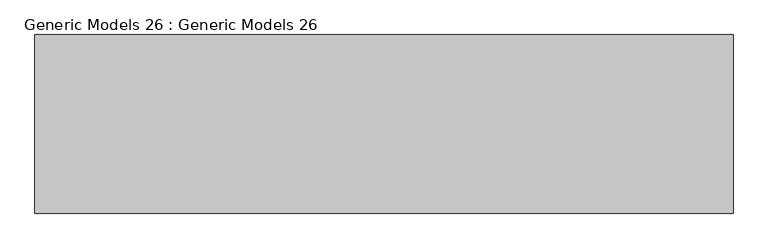
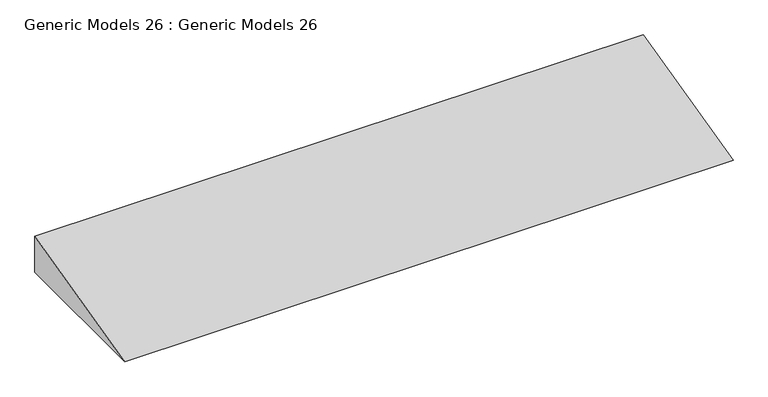
"""IFC4 building model written with IfcOpenShell, lengths in millimetres: proxy geometry, Generic Models 26 : Generic Models 26."""

from ifc_helpers import new_model, si_unit, frame, origin, place, context, project, spatial, polyline, outline, extrude, source, transform, mapped, element, save


def generic_models_26_generic_models_26_2c916a27(model_context):
    return source(origin(), model_context, "Body", "SweptSolid", [
        extrude(outline(polyline([(-7335.6844117, 0.0), (-8580.2844117, 0.0), (-7335.6844117, 304.8), (-7335.6844117, 0.0)])), frame((-4797.9586008, 0.0, 0.0), z_axis=(1.0, 0.0, 0.0), x_axis=(0.0, 1.0, 0.0)), (0.0, 0.0, 1.0), 4864.1),
    ])


if __name__ == "__main__":
    model = new_model("IFC4")
    model_context = context("Model", 3, world=origin())
    ifc_project = project(units=[si_unit("LENGTHUNIT", "METRE", prefix="MILLI")], contexts=[model_context])
    site = spatial("IfcSite", under=ifc_project)
    building = spatial("IfcBuilding", under=site)
    placement = place(None, origin())
    generic_models_26_generic_models_26_shape = generic_models_26_generic_models_26_2c916a27(model_context)
    element("IfcBuildingElementProxy", 1, Name="Generic Models 26 : Generic Models 26", ObjectType="Generic Models 26 : Generic Models 26", at=placement, inside=building, context=model_context, shape_type="MappedRepresentation", body=[
        mapped(generic_models_26_generic_models_26_shape, transform((0.0, 0.0, 0.0), x_axis=(1.0, 0.0, 0.0), y_axis=(0.0, 1.0, 0.0), z_axis=(0.0, 0.0, 1.0))),
    ])
    save(model, "model.ifc")

# Revit data of these elements
# Element 1 (IfcBuildingElementProxy, "Generic Models 26 : Generic Models 26")
#   Materials on its faces: "Concrete, Cast-in-Place gray"
# Materials
#   "Concrete, Cast-in-Place gray": class "Concrete", colour RGB 192 192 192, transparency 0, Description = "Cast-in-place concrete", Cost = 0
